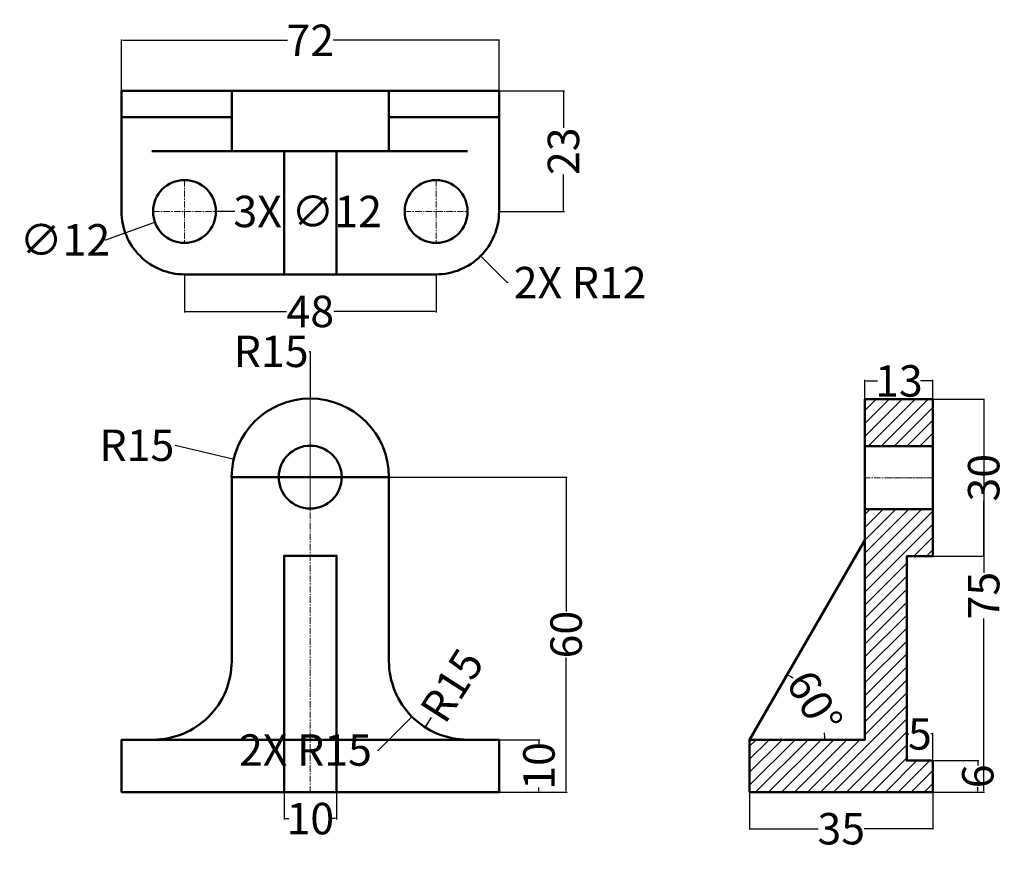
# Model space of a CAD drawing. Units: millimetres. Extents: x 68 to 256, y -8 to 151.
import ezdxf

# ---------------------------------------------------------------- set-up
doc = ezdxf.new("R2010")
doc.units = ezdxf.units.MM
doc.header["$MEASUREMENT"] = 0
doc.linetypes.add('CENTER', pattern=[2, 1.25, -0.25, 0.25, -0.25])
for name, color, linetype, lineweight in [('M-CNTR', 1, 'CENTER', 18), ('M-DIMS', 2, 'Continuous', 25), ('M-HATC', 8, 'Continuous', 18), ('M-OUTL', 7, 'Continuous', 50)]:
    doc.layers.add(name, color=color, linetype=linetype, lineweight=lineweight)
doc.styles.get("Standard").update_dxf_attribs({"font": 'arial.ttf'})
doc.dimstyles.get("Standard").update_dxf_attribs({"dimtxt": 6, "dimasz": 0.18, "dimexe": 0.18, "dimexo": 0.0625, "dimgap": 0.09, "dimtad": 0, "dimtoh": 1, "dimdec": 0, "dimzin": 0, "dimdsep": 46, "dimtxsty": 'Standard', "dimcen": 0.09, "dimadec": 0, "dimazin": 0, "dimtfac": 1, "dimtdec": 0, "dimtofl": 0, "dimtmove": 0, "dimatfit": 3, "dimfxl": 1, "dimtolj": 1, "dimtzin": 0, "dimarcsym": 0})

# ---------------------------------------------------------------- blocks, each defined once
blk = doc.blocks.new('*D1')
at = {"layer": 'Defpoints', "color": 0, "transparency": 16777216}
for p in [(105.26, 116.01), (93.97, 111.94)]:
    blk.add_point(p, dxfattribs=at)
at = {"layer": 'M-DIMS', "color": 0, "lineweight": -2, "transparency": 16777216}
for p, q in [((99.53, 113.97), (99.71, 113.97)), ((99.62, 113.88), (99.62, 114.06)), ((84.62, 108.56), (93.8, 111.87)), ((84.44, 108.56), (84.62, 108.56))]:
    blk.add_line(p, q, dxfattribs=at)
at = {"layer": 'M-DIMS', "color": 0, "transparency": 16777216}
blk.add_solid([(93.79, 111.9), (93.81, 111.85), (93.97, 111.94)], dxfattribs=at)
at = {"layer": 'M-DIMS', "color": 0, "transparency": 16777216, "insert": (76.82, 108.56), "char_height": 6, "attachment_point": 5}
blk.add_mtext('\\A1;∅12', dxfattribs=at)
blk = doc.blocks.new('*D2')
at = {"layer": 'Defpoints', "color": 0, "transparency": 16777216}
for p in [(159.62, 136.97), (159.62, 113.97), (171.91, 113.97)]:
    blk.add_point(p, dxfattribs=at)
at = {"layer": 'M-DIMS', "color": 0, "lineweight": -2, "transparency": 16777216}
for p, q in [((159.68, 136.97), (172.09, 136.97)), ((171.91, 136.79), (171.91, 129.91)), ((171.91, 114.15), (171.91, 121.03)), ((159.68, 113.97), (172.09, 113.97))]:
    blk.add_line(p, q, dxfattribs=at)
at = {"layer": 'M-DIMS', "color": 0, "transparency": 16777216}
for points in [[(171.88, 136.79), (171.94, 136.79), (171.91, 136.97)], [(171.88, 114.15), (171.94, 114.15), (171.91, 113.97)]]:
    blk.add_solid(points, dxfattribs=at)
at = {"layer": 'M-DIMS', "color": 0, "transparency": 16777216, "insert": (171.91, 125.47), "char_height": 6, "attachment_point": 5, "rotation": 90}
blk.add_mtext('\\A1;23', dxfattribs=at)
blk = doc.blocks.new('*D3')
at = {"layer": 'Defpoints', "color": 0, "transparency": 16777216}
for p in [(99.62, 101.97), (147.62, 101.97), (147.62, 94.89)]:
    blk.add_point(p, dxfattribs=at)
at = {"layer": 'M-DIMS', "color": 0, "lineweight": -2, "transparency": 16777216}
for p, q in [((99.62, 101.91), (99.62, 94.71)), ((147.62, 101.91), (147.62, 94.71)), ((99.8, 94.89), (119.1, 94.89)), ((147.44, 94.89), (128.13, 94.89))]:
    blk.add_line(p, q, dxfattribs=at)
at = {"layer": 'M-DIMS', "color": 0, "transparency": 16777216}
for points in [[(99.8, 94.92), (99.8, 94.86), (99.62, 94.89)], [(147.44, 94.92), (147.44, 94.86), (147.62, 94.89)]]:
    blk.add_solid(points, dxfattribs=at)
at = {"layer": 'M-DIMS', "color": 0, "transparency": 16777216, "insert": (123.62, 94.89), "char_height": 6, "attachment_point": 5}
blk.add_mtext('\\A1;48', dxfattribs=at)
blk = doc.blocks.new('*D4')
at = {"layer": 'Defpoints', "color": 0, "transparency": 16777216}
for p in [(159.62, 13.15), (159.62, 3.15), (167.23, 3.15)]:
    blk.add_point(p, dxfattribs=at)
at = {"layer": 'M-DIMS', "color": 0, "lineweight": -2, "transparency": 16777216}
for p, q in [((159.68, 13.15), (167.41, 13.15)), ((167.23, 12.97), (167.23, 12.24)), ((167.23, 3.33), (167.23, 4.05)), ((159.68, 3.15), (167.41, 3.15))]:
    blk.add_line(p, q, dxfattribs=at)
at = {"layer": 'M-DIMS', "color": 0, "transparency": 16777216}
for points in [[(167.2, 12.97), (167.26, 12.97), (167.23, 13.15)], [(167.2, 3.33), (167.26, 3.33), (167.23, 3.15)]]:
    blk.add_solid(points, dxfattribs=at)
at = {"layer": 'M-DIMS', "color": 0, "transparency": 16777216, "insert": (167.23, 8.15), "char_height": 6, "attachment_point": 5, "rotation": 90}
blk.add_mtext('\\A1;10', dxfattribs=at)
blk = doc.blocks.new('*D5')
at = {"layer": 'Defpoints', "color": 0, "transparency": 16777216}
for p in [(118.62, 3.15), (128.62, 3.15), (128.62, -1.91)]:
    blk.add_point(p, dxfattribs=at)
at = {"layer": 'M-DIMS', "color": 0, "lineweight": -2, "transparency": 16777216}
for p, q in [((118.62, 3.08), (118.62, -2.09)), ((128.62, 3.08), (128.62, -2.09)), ((118.8, -1.91), (119.52, -1.91)), ((128.44, -1.91), (127.71, -1.91))]:
    blk.add_line(p, q, dxfattribs=at)
at = {"layer": 'M-DIMS', "color": 0, "transparency": 16777216}
for points in [[(118.8, -1.88), (118.8, -1.94), (118.62, -1.91)], [(128.44, -1.88), (128.44, -1.94), (128.62, -1.91)]]:
    blk.add_solid(points, dxfattribs=at)
at = {"layer": 'M-DIMS', "color": 0, "transparency": 16777216, "insert": (123.62, -1.91), "char_height": 6, "attachment_point": 5}
blk.add_mtext('\\A1;10', dxfattribs=at)
blk = doc.blocks.new('*D6')
at = {"layer": 'Defpoints', "color": 0, "transparency": 16777216}
for p in [(109.02, 66.71), (123.62, 63.27)]:
    blk.add_point(p, dxfattribs=at)
at = {"layer": 'M-DIMS', "color": 0, "lineweight": -2, "transparency": 16777216}
for p, q in [((97.82, 69.35), (108.84, 66.75)), ((123.53, 63.27), (123.71, 63.27)), ((123.62, 63.18), (123.62, 63.36))]:
    blk.add_line(p, q, dxfattribs=at)
at = {"layer": 'M-DIMS', "color": 0, "transparency": 16777216}
blk.add_solid([(108.85, 66.78), (108.83, 66.72), (109.02, 66.71)], dxfattribs=at)
at = {"layer": 'M-DIMS', "color": 0, "transparency": 16777216, "insert": (90.54, 69.35), "char_height": 6, "attachment_point": 5}
blk.add_mtext('\\A1;R15', dxfattribs=at)
blk = doc.blocks.new('*D7')
at = {"layer": 'Defpoints', "color": 0, "transparency": 16777216}
for p in [(153.62, 28.15), (145.52, 15.52)]:
    blk.add_point(p, dxfattribs=at)
at = {"layer": 'M-DIMS', "color": 0, "lineweight": -2, "transparency": 16777216}
blk.add_line((146.7, 17.37), (145.62, 15.67), dxfattribs=at)
at = {"layer": 'M-DIMS', "color": 0, "transparency": 16777216}
blk.add_solid([(145.59, 15.69), (145.64, 15.65), (145.52, 15.52)], dxfattribs=at)
at = {"layer": 'M-DIMS', "color": 0, "transparency": 16777216, "insert": (150.63, 23.5), "char_height": 6, "attachment_point": 5, "rotation": 57.335}
blk.add_mtext('\\A1;R15', dxfattribs=at)
blk = doc.blocks.new('*D8')
at = {"layer": 'Defpoints', "color": 0, "transparency": 16777216}
for p in [(123.53, 63.27), (123.62, 3.15), (172.41, 3.15)]:
    blk.add_point(p, dxfattribs=at)
at = {"layer": 'M-DIMS', "color": 0, "lineweight": -2, "transparency": 16777216}
for p, q in [((123.59, 63.27), (172.59, 63.27)), ((172.41, 63.09), (172.41, 37.6)), ((172.41, 3.33), (172.41, 28.81)), ((123.68, 3.15), (172.59, 3.15))]:
    blk.add_line(p, q, dxfattribs=at)
at = {"layer": 'M-DIMS', "color": 0, "transparency": 16777216}
for points in [[(172.38, 63.09), (172.44, 63.09), (172.41, 63.27)], [(172.38, 3.33), (172.44, 3.33), (172.41, 3.15)]]:
    blk.add_solid(points, dxfattribs=at)
at = {"layer": 'M-DIMS', "color": 0, "transparency": 16777216, "insert": (172.41, 33.21), "char_height": 6, "attachment_point": 5, "rotation": 90}
blk.add_mtext('\\A1;60', dxfattribs=at)
blk = doc.blocks.new('*U9')
at = {"layer": 'M-CNTR', "color": 0, "transparency": 16777216}
blk.add_line((4.62, 0), (-4.62, 0), dxfattribs=at)
blk = doc.blocks.new('*D10')
at = {"layer": 'Defpoints', "color": 0, "transparency": 16777216}
for p in [(242.4, 81.63), (229.4, 78.15), (242.4, 78.15)]:
    blk.add_point(p, dxfattribs=at)
at = {"layer": 'M-DIMS', "color": 0, "lineweight": -2, "transparency": 16777216}
for p, q in [((229.4, 78.21), (229.4, 81.81)), ((229.58, 81.63), (231.79, 81.63)), ((242.22, 81.63), (240, 81.63)), ((242.4, 78.21), (242.4, 81.81))]:
    blk.add_line(p, q, dxfattribs=at)
at = {"layer": 'M-DIMS', "color": 0, "transparency": 16777216}
for points in [[(229.58, 81.66), (229.58, 81.6), (229.4, 81.63)], [(242.22, 81.66), (242.22, 81.6), (242.4, 81.63)]]:
    blk.add_solid(points, dxfattribs=at)
at = {"layer": 'M-DIMS', "color": 0, "transparency": 16777216, "insert": (235.9, 81.63), "char_height": 6, "attachment_point": 5}
blk.add_mtext('\\A1;13', dxfattribs=at)
blk = doc.blocks.new('*D11')
at = {"layer": 'Defpoints', "color": 0, "transparency": 16777216}
for p in [(242.4, 14.25), (237.4, 9.15), (242.4, 9.15)]:
    blk.add_point(p, dxfattribs=at)
at = {"layer": 'M-DIMS', "color": 0, "lineweight": -2, "transparency": 16777216}
for p, q in [((237.4, 9.21), (237.4, 14.43)), ((237.58, 14.25), (237.82, 14.25)), ((242.22, 14.25), (241.98, 14.25)), ((242.4, 9.21), (242.4, 14.43))]:
    blk.add_line(p, q, dxfattribs=at)
at = {"layer": 'M-DIMS', "color": 0, "transparency": 16777216}
for points in [[(237.58, 14.28), (237.58, 14.22), (237.4, 14.25)], [(242.22, 14.28), (242.22, 14.22), (242.4, 14.25)]]:
    blk.add_solid(points, dxfattribs=at)
at = {"layer": 'M-DIMS', "color": 0, "transparency": 16777216, "insert": (239.9, 14.25), "char_height": 6, "attachment_point": 5}
blk.add_mtext('\\A1;5', dxfattribs=at)
blk = doc.blocks.new('*D12')
at = {"layer": 'Defpoints', "color": 0, "transparency": 16777216}
for p in [(242.4, 9.15), (242.4, 3.15), (250.94, 3.15)]:
    blk.add_point(p, dxfattribs=at)
at = {"layer": 'M-DIMS', "color": 0, "lineweight": -2, "transparency": 16777216}
for p, q in [((242.46, 9.15), (251.12, 9.15)), ((250.94, 8.97), (250.94, 8.22)), ((250.94, 3.33), (250.94, 4.08)), ((242.46, 3.15), (251.12, 3.15))]:
    blk.add_line(p, q, dxfattribs=at)
at = {"layer": 'M-DIMS', "color": 0, "transparency": 16777216}
for points in [[(250.91, 8.97), (250.97, 8.97), (250.94, 9.15)], [(250.91, 3.33), (250.97, 3.33), (250.94, 3.15)]]:
    blk.add_solid(points, dxfattribs=at)
at = {"layer": 'M-DIMS', "color": 0, "transparency": 16777216, "insert": (250.94, 6.15), "char_height": 6, "attachment_point": 5, "rotation": 90}
blk.add_mtext('\\A1;6', dxfattribs=at)
blk = doc.blocks.new('*D13')
at = {"layer": 'Defpoints', "color": 0, "transparency": 16777216}
for p in [(207.4, 3.15), (242.4, 3.15), (242.4, -3.84)]:
    blk.add_point(p, dxfattribs=at)
at = {"layer": 'M-DIMS', "color": 0, "lineweight": -2, "transparency": 16777216}
for p, q in [((207.4, 3.08), (207.4, -4.02)), ((242.4, 3.08), (242.4, -4.02)), ((207.58, -3.84), (220.49, -3.84)), ((242.22, -3.84), (229.3, -3.84))]:
    blk.add_line(p, q, dxfattribs=at)
at = {"layer": 'M-DIMS', "color": 0, "transparency": 16777216}
for points in [[(207.58, -3.81), (207.58, -3.87), (207.4, -3.84)], [(242.22, -3.81), (242.22, -3.87), (242.4, -3.84)]]:
    blk.add_solid(points, dxfattribs=at)
at = {"layer": 'M-DIMS', "color": 0, "transparency": 16777216, "insert": (224.9, -3.84), "char_height": 6, "attachment_point": 5}
blk.add_mtext('\\A1;35', dxfattribs=at)
blk = doc.blocks.new('*D14')
at = {"layer": 'Defpoints', "color": 0, "transparency": 16777216}
for p in [(229.4, 51.25), (220.89, 18.06), (207.4, 13.15), (207.4, 13.15), (229.4, 13.15)]:
    blk.add_point(p, dxfattribs=at)
at = {"layer": 'M-DIMS', "color": 0, "lineweight": -2, "transparency": 16777216}
for start, end in [(54.6636, 59.2817), (0.7183, 5.3364)]:
    blk.add_arc((207.4, 13.15), 14.36, start, end, dxfattribs=at)
at = {"layer": 'M-DIMS', "color": 0, "transparency": 16777216}
for points in [[(214.72, 25.46), (214.75, 25.52), (214.58, 25.58)], [(221.78, 13.33), (221.72, 13.33), (221.76, 13.15)]]:
    blk.add_solid(points, dxfattribs=at)
at = {"layer": 'M-DIMS', "color": 0, "transparency": 16777216, "insert": (219.83, 20.33), "char_height": 6, "attachment_point": 5, "rotation": 300}
blk.add_mtext('\\A1;60°', dxfattribs=at)
blk = doc.blocks.new('*D15')
at = {"layer": 'Defpoints', "color": 0, "transparency": 16777216}
for p in [(159.62, 146.64), (87.62, 136.97), (159.62, 136.97)]:
    blk.add_point(p, dxfattribs=at)
at = {"layer": 'M-DIMS', "color": 0, "lineweight": -2, "transparency": 16777216}
for p, q in [((87.62, 137.04), (87.62, 146.82)), ((87.8, 146.64), (119.28, 146.64)), ((159.44, 146.64), (127.95, 146.64)), ((159.62, 137.04), (159.62, 146.82))]:
    blk.add_line(p, q, dxfattribs=at)
at = {"layer": 'M-DIMS', "color": 0, "transparency": 16777216}
for points in [[(87.8, 146.67), (87.8, 146.61), (87.62, 146.64)], [(159.44, 146.67), (159.44, 146.61), (159.62, 146.64)]]:
    blk.add_solid(points, dxfattribs=at)
at = {"layer": 'M-DIMS', "color": 0, "transparency": 16777216, "insert": (123.62, 146.64), "char_height": 6, "attachment_point": 5}
blk.add_mtext('\\A1;72', dxfattribs=at)
blk = doc.blocks.new('*D16')
at = {"layer": 'Defpoints', "color": 0, "transparency": 16777216}
for p in [(242.4, 78.15), (252.07, 78.15), (242.4, 3.15)]:
    blk.add_point(p, dxfattribs=at)
at = {"layer": 'M-DIMS', "color": 0, "lineweight": -2, "transparency": 16777216}
for p, q in [((242.46, 78.15), (252.25, 78.15)), ((252.07, 77.97), (252.07, 45.03)), ((252.07, 3.33), (252.07, 36.26)), ((242.46, 3.15), (252.25, 3.15))]:
    blk.add_line(p, q, dxfattribs=at)
at = {"layer": 'M-DIMS', "color": 0, "transparency": 16777216}
for points in [[(252.04, 77.97), (252.1, 77.97), (252.07, 78.15)], [(252.04, 3.33), (252.1, 3.33), (252.07, 3.15)]]:
    blk.add_solid(points, dxfattribs=at)
at = {"layer": 'M-DIMS', "color": 0, "transparency": 16777216, "insert": (252.07, 40.65), "char_height": 6, "attachment_point": 5, "rotation": 90}
blk.add_mtext('\\A1;75', dxfattribs=at)
blk = doc.blocks.new('*D17')
at = {"layer": 'Defpoints', "color": 0, "transparency": 16777216}
for p in [(242.4, 78.15), (252.07, 78.15), (237.4, 48.15)]:
    blk.add_point(p, dxfattribs=at)
at = {"layer": 'M-DIMS', "color": 0, "lineweight": -2, "transparency": 16777216}
for p, q in [((242.46, 78.15), (252.25, 78.15)), ((252.07, 77.97), (252.07, 67.52)), ((252.07, 48.33), (252.07, 58.77)), ((237.46, 48.15), (252.25, 48.15))]:
    blk.add_line(p, q, dxfattribs=at)
at = {"layer": 'M-DIMS', "color": 0, "transparency": 16777216}
for points in [[(252.04, 77.97), (252.1, 77.97), (252.07, 78.15)], [(252.04, 48.33), (252.1, 48.33), (252.07, 48.15)]]:
    blk.add_solid(points, dxfattribs=at)
at = {"layer": 'M-DIMS', "color": 0, "transparency": 16777216, "insert": (252.07, 63.15), "char_height": 6, "attachment_point": 5, "rotation": 90}
blk.add_mtext('\\A1;30', dxfattribs=at)
blk = doc.blocks.new('*D18')
at = {"layer": 'Defpoints', "color": 0, "transparency": 16777216}
for p in [(147.62, 113.97), (156.1, 105.49)]:
    blk.add_point(p, dxfattribs=at)
at = {"layer": 'M-DIMS', "color": 0, "lineweight": -2, "transparency": 16777216}
for p, q in [((147.53, 113.97), (147.71, 113.97)), ((147.62, 113.88), (147.62, 114.06)), ((161.19, 100.4), (156.23, 105.36)), ((161.37, 100.4), (161.19, 100.4))]:
    blk.add_line(p, q, dxfattribs=at)
at = {"layer": 'M-DIMS', "color": 0, "transparency": 16777216}
blk.add_solid([(156.25, 105.38), (156.21, 105.34), (156.1, 105.49)], dxfattribs=at)
at = {"layer": 'M-DIMS', "color": 0, "transparency": 16777216, "insert": (175.1, 100.4), "char_height": 6, "attachment_point": 5}
blk.add_mtext('\\A1;2X R12', dxfattribs=at)
blk = doc.blocks.new('*D19')
at = {"layer": 'Defpoints', "color": 0, "transparency": 16777216}
for p in [(123.61, 78.27), (123.61, 63.27)]:
    blk.add_point(p, dxfattribs=at)
at = {"layer": 'M-DIMS', "color": 0, "lineweight": -2, "transparency": 16777216}
for p, q in [((123.43, 87.27), (123.61, 87.27)), ((123.61, 87.27), (123.61, 78.45)), ((123.53, 63.27), (123.71, 63.27)), ((123.61, 63.18), (123.61, 63.36))]:
    blk.add_line(p, q, dxfattribs=at)
at = {"layer": 'M-DIMS', "color": 0, "transparency": 16777216}
blk.add_solid([(123.64, 78.45), (123.58, 78.45), (123.61, 78.27)], dxfattribs=at)
at = {"layer": 'M-DIMS', "color": 0, "transparency": 16777216, "insert": (116.15, 87.27), "char_height": 6, "attachment_point": 5}
blk.add_mtext('\\A1;R15', dxfattribs=at)
blk = doc.blocks.new('*D20')
at = {"layer": 'Defpoints', "color": 0, "transparency": 16777216}
for p in [(153.62, 28.15), (143.01, 17.54)]:
    blk.add_point(p, dxfattribs=at)
at = {"layer": 'M-DIMS', "color": 0, "lineweight": -2, "transparency": 16777216}
for p, q in [((153.62, 28.06), (153.62, 28.24)), ((153.53, 28.15), (153.71, 28.15)), ((136.64, 11.18), (142.88, 17.41)), ((136.46, 11.18), (136.64, 11.18))]:
    blk.add_line(p, q, dxfattribs=at)
at = {"layer": 'M-DIMS', "color": 0, "transparency": 16777216}
blk.add_solid([(142.86, 17.43), (142.9, 17.39), (143.01, 17.54)], dxfattribs=at)
at = {"layer": 'M-DIMS', "color": 0, "transparency": 16777216, "insert": (122.69, 11.18), "char_height": 6, "attachment_point": 5}
blk.add_mtext('\\A1;2X R15', dxfattribs=at)
blk = doc.blocks.new('*D21')
at = {"layer": 'Defpoints', "color": 0, "transparency": 16777216}
for p in [(93.62, 113.97), (105.62, 113.97)]:
    blk.add_point(p, dxfattribs=at)
at = {"layer": 'M-DIMS', "color": 0, "lineweight": -2, "transparency": 16777216}
for p, q in [((99.53, 113.97), (99.71, 113.97)), ((99.62, 113.88), (99.62, 114.06)), ((109.22, 113.97), (105.8, 113.97))]:
    blk.add_line(p, q, dxfattribs=at)
at = {"layer": 'M-DIMS', "color": 0, "transparency": 16777216}
blk.add_solid([(105.8, 114), (105.8, 113.94), (105.62, 113.97)], dxfattribs=at)
at = {"layer": 'M-DIMS', "color": 0, "transparency": 16777216, "insert": (123.12, 113.97), "char_height": 6, "attachment_point": 5}
blk.add_mtext('\\A1;3X ∅12', dxfattribs=at)

msp = doc.modelspace()

# ---------------------------------------------------------------- hatches: boundary and pattern name
at = {"layer": 'M-HATC'}
h = msp.add_hatch(dxfattribs=at)
h.set_pattern_fill('ANSI31', color=256, scale=14)
h.paths.add_polyline_path([(242.4, 78.15), (229.4, 78.15), (229.4, 69.15), (242.4, 69.15)])
h.paths.add_polyline_path([(242.4, 57.15), (229.4, 57.15), (229.4, 13.15), (207.4, 13.15), (207.4, 3.15), (242.4, 3.15), (242.4, 9.15), (237.4, 9.15), (237.4, 48.15), (242.4, 48.15)])

# ---------------------------------------------------------------- linework, layer by layer
at = {"layer": 'M-CNTR'}
for p, q in [((99.62, 119.97), (99.62, 107.97)), ((147.62, 119.97), (147.62, 107.97)), ((93.62, 113.97), (105.62, 113.97)), ((141.62, 113.97), (153.62, 113.97)), ((242.4, 63.15), (229.4, 63.15))]:
    msp.add_line(p, q, dxfattribs=at)
msp.add_lwpolyline([(123.61, 3.03), (123.61, 13.27), (123.61, 63.27), (123.61, 78.27), (123.61, 57.27)], dxfattribs=at)
at = {"layer": 'M-OUTL'}
for p, q in [((108.62, 137.09), (108.62, 125.47)), ((118.62, 137.09), (118.62, 136.97)), ((128.62, 137.09), (128.62, 136.97)), ((138.62, 137.09), (138.62, 125.47)), ((87.62, 131.97), (108.62, 131.97)), ((159.62, 131.97), (138.62, 131.97)), ((118.62, 125.47), (118.62, 101.97)), ((128.62, 125.47), (128.62, 101.97)), ((242.4, 69.15), (229.4, 69.15)), ((242.4, 57.15), (229.4, 57.15)), ((118.62, 13.15), (118.62, 48.27)), ((118.62, 3.03), (118.62, 13.27)), ((128.62, 3.15), (128.62, 13.15))]:
    msp.add_line(p, q, dxfattribs=at)
msp.add_lwpolyline([(87.62, 136.97), (87.62, 113.97, 0.414214), (99.62, 101.97), (147.62, 101.97, 0.414214), (159.62, 113.97), (159.62, 113.97), (159.62, 136.97)], format="xyb", close=True, dxfattribs=at)
msp.add_lwpolyline([(123.61, 137.09), (123.61, 136.97)], close=True, dxfattribs=at)
for points in [[(93.39, 125.47), (118.62, 125.47), (128.62, 125.47), (153.62, 125.47)], [(207.4, 13.15), (229.4, 13.15), (229.4, 78.15), (242.4, 78.15), (242.4, 48.15), (237.4, 48.15), (237.4, 9.15), (242.4, 9.15), (242.4, 3.15), (207.4, 3.15), (207.4, 13.15), (207.4, 13.15), (229.4, 51.25)], [(123.61, 48.27), (118.62, 48.27), (128.62, 48.27), (128.62, 13.27), (128.62, 13.15)], [(128.62, 3.15), (128.62, 3.03)]]:
    msp.add_lwpolyline(points, dxfattribs=at)
msp.add_lwpolyline([(153.62, 13.15, -0.414214), (138.62, 28.15), (138.62, 63.27), (108.62, 63.27), (108.62, 28.15, -0.414214), (93.62, 13.15), (153.62, 13.15), (159.62, 13.15), (159.62, 3.15), (87.62, 3.15), (87.62, 13.15), (93.62, 13.15)], format="xyb", dxfattribs=at)
for centre in [(99.62, 113.97), (147.62, 113.97), (123.61, 63.27)]:
    msp.add_circle(centre, 6, dxfattribs=at)
msp.add_arc((123.61, 63.27), 15, 360, 180, dxfattribs=at)

# ---------------------------------------------------------------- block references
at = {"layer": 'M-CNTR'}
msp.add_blockref('*U9', (237.9, 63.15), dxfattribs=at)

# ---------------------------------------------------------------- dimensions: what is measured, and where the dimension line sits
at = {"layer": 'M-DIMS'}
for base, p1, p2, override, picture, middle in [((159.62, 146.64), (87.62, 136.97), (159.62, 136.97), {"dimdec": 0, "dimlfac": 1, "dimrnd": 0, "dimzin": 0, "dimdsep": 46, "dimlunit": 2}, '*D15', (123.61, 146.64)), ((147.62, 94.89), (99.62, 101.97), (147.62, 101.97), {"dimclrd": 0, "dimclre": 0, "dimclrt": 0}, '*D3', (123.61, 94.89)), ((242.4, 81.63), (229.4, 78.15), (242.4, 78.15), {"dimclrd": 0, "dimclre": 0, "dimclrt": 0}, '*D10', (235.9, 81.63)), ((242.4, 14.25), (237.4, 9.15), (242.4, 9.15), {"dimclrd": 0, "dimclre": 0, "dimclrt": 0}, '*D11', (239.9, 14.25)), ((128.62, -1.91), (118.62, 3.15), (128.62, 3.15), {"dimclrd": 0, "dimclre": 0, "dimclrt": 0}, '*D5', (123.61, -1.91)), ((242.4, -3.84), (207.4, 3.15), (242.4, 3.15), {"dimclrd": 0, "dimclre": 0, "dimclrt": 0}, '*D13', (224.9, -3.84))]:
    dim = msp.add_linear_dim(base=base, p1=p1, p2=p2, dimstyle='Standard', override=override, dxfattribs=at)
    dim.commit()
    dim.dimension.update_dxf_attribs({"geometry": picture, "text_midpoint": middle})
for base, p1, p2, override, picture, middle in [((171.91, 113.97), (159.62, 136.97), (159.62, 113.97), {"dimclrd": 0, "dimclre": 0, "dimclrt": 0}, '*D2', (171.91, 125.47)), ((252.07, 78.15), (237.4, 48.15), (242.4, 78.15), {"dimdec": 0, "dimlfac": 1, "dimrnd": 0, "dimzin": 0, "dimdsep": 46, "dimlunit": 2}, '*D17', (252.07, 63.15)), ((252.07, 78.15), (242.4, 3.15), (242.4, 78.15), {"dimdec": 0, "dimlfac": 1, "dimrnd": 0, "dimzin": 0, "dimdsep": 46, "dimlunit": 2}, '*D16', (252.07, 40.65)), ((172.41, 3.15), (123.53, 63.27), (123.61, 3.15), {"dimclrd": 0, "dimclre": 0, "dimclrt": 0}, '*D8', (172.41, 33.21)), ((167.23, 3.15), (159.62, 13.15), (159.62, 3.15), {"dimclrd": 0, "dimclre": 0, "dimclrt": 0}, '*D4', (167.23, 8.15)), ((250.94, 3.15), (242.4, 9.15), (242.4, 3.15), {"dimclrd": 0, "dimclre": 0, "dimclrt": 0}, '*D12', (250.94, 6.15))]:
    dim = msp.add_linear_dim(base=base, p1=p1, p2=p2, angle=90, dimstyle='Standard', override=override, dxfattribs=at)
    dim.commit()
    dim.dimension.update_dxf_attribs({"geometry": picture, "text_midpoint": middle})
dim = msp.add_diameter_dim_2p(p1=(93.62, 113.97), p2=(105.62, 113.97), text='3X <>', dimstyle='Standard', override={"dimdec": 0, "dimlfac": 1, "dimrnd": 0, "dimzin": 0, "dimdsep": 46, "dimlunit": 2}, dxfattribs=at)
dim.commit()
dim.dimension.update_dxf_attribs({"geometry": '*D21', "text_midpoint": (109.22, 113.97), "dimtype": 163})
dim = msp.add_diameter_dim_2p(p1=(105.26, 116.01), p2=(93.97, 111.94), dimstyle='Standard', override={"dimclrd": 0, "dimclre": 0, "dimclrt": 0}, dxfattribs=at)
dim.commit()
dim.dimension.update_dxf_attribs({"geometry": '*D1', "text_midpoint": (76.82, 108.56), "dimtype": 163})
for center, mpoint, picture, middle in [((147.62, 113.97), (156.1, 105.49), '*D18', (175.1, 100.4)), ((153.62, 28.15), (143.01, 17.54), '*D20', (122.69, 11.18))]:
    dim = msp.add_radius_dim(center=center, mpoint=mpoint, text='2X <>', dimstyle='Standard', override={"dimdec": 0, "dimlfac": 1, "dimrnd": 0, "dimzin": 0, "dimdsep": 46, "dimlunit": 2}, dxfattribs=at)
    dim.commit()
    dim.dimension.update_dxf_attribs({"geometry": picture, "text_midpoint": middle, "dimtype": 164})
for center, mpoint, override, picture, middle in [((123.61, 63.27), (123.61, 78.27), {"dimdec": 0, "dimlfac": 1, "dimrnd": 0, "dimzin": 0, "dimdsep": 46, "dimlunit": 2}, '*D19', (116.15, 87.27)), ((123.61, 63.27), (109.02, 66.71), {"dimclrd": 0, "dimclre": 0, "dimclrt": 0}, '*D6', (97.82, 69.35)), ((153.62, 28.15), (145.52, 15.52), {"dimclrd": 0, "dimclre": 0, "dimclrt": 0}, '*D7', (150.63, 23.5))]:
    dim = msp.add_radius_dim(center=center, mpoint=mpoint, dimstyle='Standard', override=override, dxfattribs=at)
    dim.commit()
    dim.dimension.update_dxf_attribs({"geometry": picture, "text_midpoint": middle, "dimtype": 164})
dim = msp.add_angular_dim_2l(base=(220.89, 18.06), line1=((207.4, 13.15), (229.4, 13.15)), line2=((207.4, 13.15), (229.4, 51.25)), dimstyle='Standard', override={"dimclrd": 0, "dimclre": 0, "dimclrt": 0}, dxfattribs=at)
dim.commit()
dim.dimension.update_dxf_attribs({"geometry": '*D14', "text_midpoint": (219.83, 20.33)})

doc.saveas('drawing.dxf')
